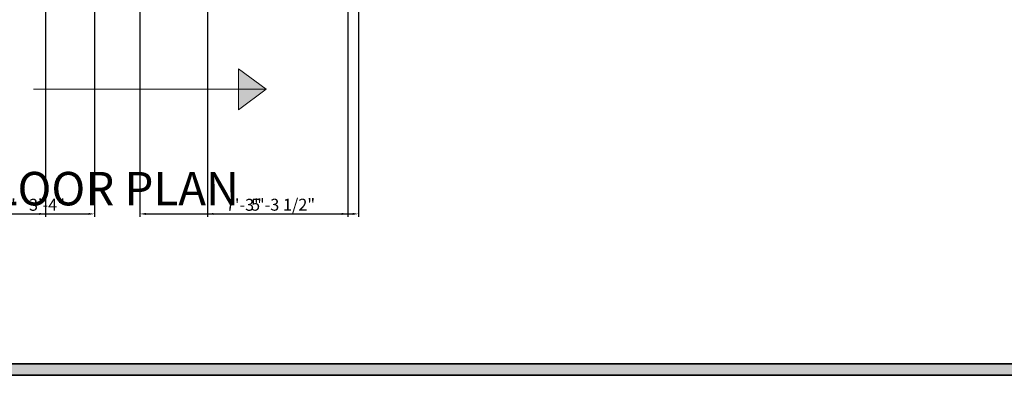
# Model space of a CAD drawing. Units: inches. Extents: x 1804 to 3296, y 909 to 2477.
# Tile 5 of 31: x 2130 to 2543, y 909 to 1059. Entities that reach past the tile are written whole.
import ezdxf

# ---------------------------------------------------------------- set-up
doc = ezdxf.new("R2010")
doc.units = ezdxf.units.IN
for name, color, linetype, lineweight in [('A-ANNO-DIMS', 2, 'Continuous', 18), ('A-ANNO-SYMB', 7, 'Continuous', 18), ('A-ANNO-TTLB', 156, 'Continuous', 35), ('A-WALL-PATT', 10, 'Continuous', 13), ('TEXT', 190, 'Continuous', 18)]:
    doc.layers.add(name, color=color, linetype=linetype, lineweight=lineweight)
doc.styles.get("Standard").update_dxf_attribs({"font": 'arial.ttf'})
doc.dimstyles.new('ISO-25', dxfattribs={"dimtxt": 5, "dimasz": 2.5, "dimexe": 1.25, "dimexo": 0.625, "dimtad": 1, "dimdec": 0, "dimlunit": 4, "dimtxsty": 'Standard', "dimcen": 2.5, "dimadec": 0, "dimazin": 0, "dimtfac": 1, "dimtdec": 0, "dimtmove": 0, "dimatfit": 3, "dimfxl": 1, "dimarcsym": 0})

# ---------------------------------------------------------------- blocks, each defined once
blk = doc.blocks.new('ROAD-DIRECTION')
h = blk.add_hatch(color=256)
h.dxf.hatch_style = 1
h.paths.add_polyline_path([(11.63, 8.56), (0, 8.56), (11.63, 0)])
h.paths.add_polyline_path([(11.63, 17.12), (0, 8.56), (11.63, 8.56)])
for p, q in [((0, 8.56), (11.63, 17.12)), ((11.63, 0), (11.63, 17.12)), ((97.65, 8.56), (0, 8.56)), ((0, 8.56), (11.63, 0))]:
    blk.add_line(p, q)
blk = doc.blocks.new('*D56')
at = {"layer": 'A-ANNO-DIMS', "color": 0, "lineweight": -2, "transparency": 16777216}
for p, q in [((2180.87, 1680.42), (2180.87, 975.89)), ((2268, 1680.42), (2268, 975.89)), ((2183.37, 977.14), (2265.5, 977.14))]:
    blk.add_line(p, q, dxfattribs=at)
at = {"layer": 'A-ANNO-DIMS', "color": 0, "lineweight": 100, "transparency": 16777216}
for points in [[(2183.37, 977.56), (2183.37, 976.72), (2180.87, 977.14)], [(2265.5, 977.56), (2265.5, 976.72), (2268, 977.14)]]:
    blk.add_solid(points, dxfattribs=at)
at = {"layer": 'Defpoints', "color": 0, "lineweight": 100, "transparency": 16777216}
for p in [(2180.87, 1681.04), (2268, 1681.04), (2268, 977.14)]:
    blk.add_point(p, dxfattribs=at)
at = {"layer": 'A-ANNO-DIMS', "color": 0, "transparency": 16777216, "insert": (2224.44, 980.32), "char_height": 5, "attachment_point": 5}
blk.add_mtext('7\'-3"', dxfattribs=at)
blk = doc.blocks.new('*D59')
at = {"layer": 'A-ANNO-DIMS', "color": 0, "lineweight": -2, "transparency": 16777216}
for p, q in [((2121.83, 1590.3), (2121.83, 975.89)), ((2161.83, 1590.3), (2161.83, 975.89)), ((2124.33, 977.14), (2159.33, 977.14))]:
    blk.add_line(p, q, dxfattribs=at)
at = {"layer": 'A-ANNO-DIMS', "color": 0, "lineweight": 100, "transparency": 16777216}
for points in [[(2124.33, 977.56), (2124.33, 976.72), (2121.83, 977.14)], [(2159.33, 977.56), (2159.33, 976.72), (2161.83, 977.14)]]:
    blk.add_solid(points, dxfattribs=at)
at = {"layer": 'Defpoints', "color": 0, "lineweight": 100, "transparency": 16777216}
for p in [(2121.83, 1590.92), (2161.83, 1590.92), (2161.83, 977.14)]:
    blk.add_point(p, dxfattribs=at)
at = {"layer": 'A-ANNO-DIMS', "color": 0, "transparency": 16777216, "insert": (2141.83, 980.32), "char_height": 5, "attachment_point": 5}
blk.add_mtext('3\'-4"', dxfattribs=at)
blk = doc.blocks.new('*D61')
at = {"layer": 'A-ANNO-DIMS', "color": 0, "lineweight": -2, "transparency": 16777216}
for p, q in [((2101.21, 1137.44), (2101.21, 975.89)), ((2141.21, 1137.44), (2141.21, 975.89)), ((2103.71, 977.14), (2138.71, 977.14))]:
    blk.add_line(p, q, dxfattribs=at)
at = {"layer": 'A-ANNO-DIMS', "color": 0, "lineweight": 100, "transparency": 16777216}
for points in [[(2103.71, 977.56), (2103.71, 976.72), (2101.21, 977.14)], [(2138.71, 977.56), (2138.71, 976.72), (2141.21, 977.14)]]:
    blk.add_solid(points, dxfattribs=at)
at = {"layer": 'Defpoints', "color": 0, "lineweight": 100, "transparency": 16777216}
for p in [(2101.21, 1138.07), (2141.21, 1138.07), (2141.21, 977.14)]:
    blk.add_point(p, dxfattribs=at)
at = {"layer": 'A-ANNO-DIMS', "color": 0, "transparency": 16777216, "insert": (2121.21, 980.32), "char_height": 5, "attachment_point": 5}
blk.add_mtext('3\'-4"', dxfattribs=at)
blk = doc.blocks.new('*D69')
at = {"layer": 'A-ANNO-DIMS', "color": 0, "lineweight": -2, "transparency": 16777216}
for p, q in [((2209.19, 1223.01), (2209.19, 975.89)), ((2272.59, 1223.01), (2272.59, 975.89)), ((2211.69, 977.14), (2270.09, 977.14))]:
    blk.add_line(p, q, dxfattribs=at)
at = {"layer": 'A-ANNO-DIMS', "color": 0, "lineweight": 100, "transparency": 16777216}
for points in [[(2211.69, 977.56), (2211.69, 976.72), (2209.19, 977.14)], [(2270.09, 977.56), (2270.09, 976.72), (2272.59, 977.14)]]:
    blk.add_solid(points, dxfattribs=at)
at = {"layer": 'Defpoints', "color": 0, "lineweight": 100, "transparency": 16777216}
for p in [(2209.19, 1223.63), (2272.59, 1223.63), (2272.59, 977.14)]:
    blk.add_point(p, dxfattribs=at)
at = {"layer": 'A-ANNO-DIMS', "color": 0, "transparency": 16777216, "insert": (2240.89, 980.35), "char_height": 5, "attachment_point": 5}
blk.add_mtext('5\'-3 1/2"', dxfattribs=at)

msp = doc.modelspace()

# ---------------------------------------------------------------- hatches: boundary and pattern name
at = {"layer": 'A-ANNO-TTLB'}
h = msp.add_hatch(color=256, dxfattribs=at)
h.dxf.hatch_style = 1
h.paths.add_polyline_path([(3294.53, 2476.54), (1803.79, 2476.54), (1805.43, 909.47), (3296.17, 909.47)])
h.paths.add_polyline_path([(1811, 914.33), (1812.79, 2467.54), (3285.53, 2467.54), (3283.74, 914.33)], flags=16)
h.paths.add_polyline_path([(1925.58, 1062.77), (1925.58, 1138.07), (1925.58, 1539.88), (1925.58, 1793.38), (1925.58, 1830.04), (2325.54, 1830.04), (2325.54, 1793.38), (2325.54, 1586.42), (2325.54, 1138.07), (2325.54, 1062.77)], flags=0)
h.paths.add_polyline_path([(1997.22, 1029.4), (2008.85, 1037.96), (2008.85, 1020.84)], flags=0)
h.paths.add_polyline_path([(1934.58, 1138.07), (1934.58, 1147.07), (2078.77, 1147.07), (2078.77, 1138.07), (2060.94, 1138.07)], flags=0)
h.paths.add_polyline_path([(1944.35, 1138.07), (1944.35, 1147.07), (2056.05, 1147.07), (2056.05, 1138.07)], flags=0)
h.paths.add_polyline_path([(2222.24, 1037.96), (2233.87, 1029.4), (2222.24, 1020.84)], flags=0)
h.paths.add_polyline_path([(2061.94, 1139.07), (2061.94, 1146.07), (2077.77, 1146.07), (2077.77, 1139.07)], flags=0)
h.paths.add_polyline_path([(2149.58, 1138.07), (2149.58, 1269.44), (2158.58, 1269.44), (2158.58, 1326.69), (2149.58, 1326.69), (2149.58, 1340.94), (2139.6, 1340.94), (2139.6, 1434.25), (2149.58, 1434.25), (2149.58, 1447.36), (2158.58, 1447.36), (2158.58, 1423.87), (2158.58, 1408.06), (2198.46, 1408.06), (2198.46, 1412.56), (2282.65, 1412.56), (2282.65, 1465.94), (2316.54, 1465.94), (2316.54, 1590.92), (2192.86, 1590.92), (2192.86, 1595.3), (2291.17, 1595.3), (2291.17, 1590.92), (2316.54, 1590.92), (2316.54, 1784.38), (2300.24, 1784.38), (2300.24, 1757.47), (2268, 1757.47), (2268, 1681.04), (2180.87, 1681.04), (2180.87, 1757.47), (2148.63, 1757.47), (2148.63, 1784.38), (2119.08, 1784.38), (2119.08, 1585.58), (2114.58, 1585.58), (2114.58, 1784.38), (2064.11, 1784.38), (2046.28, 1784.38), (2046.28, 1760.38), (1958.58, 1760.38), (1958.58, 1664.38), (1934.58, 1664.38), (1934.58, 1784.38), (1934.58, 1793.38), (2046.28, 1793.38), (2064.11, 1793.38), (2119.08, 1793.38), (2230.78, 1793.38), (2230.78, 1784.38), (2268, 1784.38), (2300.24, 1784.38), (2316.54, 1784.38), (2316.54, 1590.92), (2316.54, 1373.73), (2316.54, 1138.07)], flags=0)
h.paths.add_polyline_path([(2209.19, 1166.63), (2209.19, 1175.63), (2158.58, 1175.63), (2209.19, 1223.63), (2209.19, 1231.63), (2183.88, 1231.63), (2183.88, 1301.66), (2242.59, 1301.66), (2242.59, 1326.69), (2316.54, 1326.69), (2272.59, 1271.63), (2272.59, 1223.63), (2316.54, 1175.63), (2272.59, 1175.63), (2272.59, 1166.63)], flags=0)
h.paths.add_polyline_path([(1947.77, 1345.22), (1947.77, 1457.48), (1991.2, 1457.48), (1991.2, 1451.7), (1991.2, 1352.18), (1991.2, 1345.22)], flags=0)
h.paths.add_polyline_path([(2209.19, 1271.63), (2262.59, 1271.63), (2262.59, 1311.85), (2272.59, 1301.66), (2272.59, 1271.63), (2269.92, 1269.63), (2270.59, 1269.63), (2270.59, 1225.63), (2211.19, 1225.63), (2211.19, 1269.63), (2211.86, 1269.63)], flags=0)
h.paths.add_polyline_path([(2000.34, 1378.21), (2000.34, 1429.71), (2025.22, 1429.71), (2025.22, 1378.21)], flags=0)
h.paths.add_polyline_path([(2001.34, 1379.21), (2001.34, 1428.71), (2024.22, 1428.71), (2024.22, 1379.21)], flags=0)
h.paths.add_polyline_path([(2012.34, 1390.21), (2012.34, 1417.71), (2013.22, 1417.71), (2013.22, 1390.21)], flags=0)
h.paths.add_polyline_path([(2237.56, 1331.19), (2237.56, 1340.18), (2238.62, 1340.18), (2238.62, 1386.84), (2241.04, 1386.84), (2242.06, 1386.84), (2242.06, 1408.06), (2316.54, 1331.19)], flags=0)
h.paths.add_polyline_path([(1953.73, 1464.35), (1953.73, 1498.59), (1981.74, 1498.59), (1981.74, 1464.35)], flags=0)
h.paths.add_polyline_path([(1987.63, 1462.08), (1987.63, 1500.95), (2104.07, 1500.95), (2104.07, 1462.08), (2099.27, 1462.08), (1993.6, 1462.08)], flags=0)
h.paths.add_polyline_path([(1956.06, 1481.47, -1), (1979.41, 1481.47, -1)], flags=0)
edge = h.paths.add_edge_path(flags=0)
edge.add_ellipse((2299.53, 1438.37), major_axis=(0.31, 21.36), ratio=0.670333, start_angle=0, end_angle=360)
h.paths.add_polyline_path([(2297.39, 1438.37, -1), (2301.67, 1438.37, -1)], flags=0)
h.paths.add_polyline_path([(2591.54, 1163.23), (2591.54, 1179.38), (2591.54, 1379.68), (2591.54, 1395.84), (2734.5, 1395.84), (2734.5, 1379.68), (2734.5, 1179.38), (2734.5, 1163.23)], flags=0)
h.paths.add_polyline_path([(2592.54, 1164.23), (2592.54, 1166.23), (2733.5, 1166.23), (2733.5, 1164.23)], flags=0)
h.paths.add_polyline_path([(2592.54, 1180.38), (2592.54, 1378.68), (2733.5, 1378.68), (2733.5, 1180.38)], flags=0)
h.paths.add_polyline_path([(2593.54, 1181.38), (2593.54, 1377.68), (2732.5, 1377.68), (2732.5, 1181.38)], flags=0)
h.paths.add_polyline_path([(2594.54, 1182.38), (2594.54, 1376.68), (2731.5, 1376.68), (2731.5, 1182.38)], flags=0)
h.paths.add_polyline_path([(1936.95, 1697.46), (1936.95, 1736.46), (1955.41, 1736.46), (1955.41, 1697.46)], flags=0)
h.paths.add_polyline_path([(1938.48, 1718.36), (1938.48, 1734.92), (1953.65, 1734.92), (1953.65, 1718.36)], flags=0)
h.paths.add_polyline_path([(1944.75, 1726.64, -1), (1947.37, 1726.64, -1)], flags=0)
h.paths.add_polyline_path([(2592.54, 1394.84), (2733.5, 1394.84), (2733.5, 1392.84), (2592.54, 1392.84)], flags=0)
h.paths.add_polyline_path([(1976.61, 1762.5), (1976.61, 1781.44), (2012.79, 1781.44), (2012.79, 1762.5)], flags=0)
h.paths.add_polyline_path([(1979.57, 1771.97, -1), (1991.39, 1771.97, -1)], flags=0)
h.paths.add_polyline_path([(1995.36, 1771.97, -1), (2007.18, 1771.97, -1)], flags=0)
h.paths.add_polyline_path([(2251.51, 1744.53), (2268, 1730.05), (2251.51, 1730.05)], flags=0)
h.paths.add_polyline_path([(2047.28, 1785.38), (2047.28, 1792.38), (2063.11, 1792.38), (2063.11, 1785.38)], flags=0)
h.paths.add_polyline_path([(2155.08, 1770.92, -1), (2174.42, 1770.92, -1)], flags=0)
h.paths.add_polyline_path([(2188.59, 1758.27), (2188.59, 1772.81), (2222.3, 1772.81), (2222.3, 1758.27)], flags=0)
h.paths.add_polyline_path([(2223.97, 1758.27), (2223.97, 1772.81), (2257.68, 1772.81), (2257.68, 1758.27)], flags=0)
h.paths.add_polyline_path([(2274.45, 1770.92, -1), (2293.8, 1770.92, -1)], flags=0)
h.paths.add_polyline_path([(2591.54, 1582.09), (2591.54, 1782.39), (2734.5, 1782.39), (2734.5, 1582.09)], flags=0)
h.paths.add_polyline_path([(2592.54, 1583.09), (2592.54, 1781.39), (2733.5, 1781.39), (2733.5, 1583.09)], flags=0)
h.paths.add_polyline_path([(2593.54, 1584.09), (2593.54, 1780.39), (2732.5, 1780.39), (2732.5, 1584.09)], flags=0)
h.paths.add_polyline_path([(2594.54, 1585.09), (2594.54, 1779.39), (2731.5, 1779.39), (2731.5, 1585.09)], flags=0)
h.paths.add_polyline_path([(1922.17, 1978.79), (1922.17, 2295.08), (1922.17, 2296.08), (2115.67, 2296.08), (2115.67, 2384.31), (2115.67, 2385.31), (2322.12, 2385.31), (2323.12, 2385.31), (2323.12, 1979.79), (2323.12, 1978.79), (1923.17, 1978.79)], flags=0)
h.paths.add_polyline_path([(1922.17, 1978.79), (1922.17, 2051.31), (1922.17, 2214.86), (1922.17, 2296.08), (2115.67, 2296.08), (2115.67, 2385.31), (2323.12, 2385.31), (2323.12, 2280.42), (2323.12, 1978.79), (2115.67, 1978.79)], flags=0)
h.paths.add_polyline_path([(1923.17, 1979.79), (1923.17, 2050.31), (2115.67, 2050.31), (2115.67, 2051.31), (1923.17, 2051.31), (1923.17, 2213.86), (1923.17, 2214.86), (1923.17, 2295.08), (1990.02, 2295.08), (1990.02, 2214.86), (1991.02, 2214.86), (1991.02, 2295.08), (2115.67, 2295.08), (2115.67, 1979.79), (2116.67, 1979.79), (2116.67, 2304.18), (2116.67, 2384.31), (2322.12, 2384.31), (2322.12, 2280.42), (2322.12, 1979.79), (2115.67, 1979.79)], flags=0)
h.paths.add_polyline_path([(2972.46, 1192.5), (2972.46, 1196.92), (2995.47, 1196.92), (2995.47, 1255.47), (2995.09, 1255.47), (2987.42, 1249.39), (2980.08, 1255.47), (2978.05, 1255.47), (2978.05, 1257.24), (2995.47, 1257.24), (2995.47, 1261.58), (3015.37, 1261.58), (3015.37, 1333.28), (3015.37, 1414.4), (3032.82, 1414.4), (3032.82, 1333.28), (3032.82, 1261.58), (3052.66, 1261.58), (3052.66, 1255.47), (3079.86, 1255.47), (3078.72, 1254.57), (3081.47, 1252.29), (3078.56, 1249.99), (3075.81, 1252.26), (3072.57, 1249.69), (3070.36, 1251.52), (3067.67, 1249.39), (3060.34, 1255.47), (3052.66, 1255.47), (3052.66, 1196.92), (3054.58, 1196.92), (3074, 1196.92), (3074, 1192.5), (3052.66, 1192.5), (2995.47, 1192.5)], flags=0)
h.paths.add_polyline_path([(2490.75, 1979.27), (2490.75, 1980.27), (2596.87, 1980.27), (2596.87, 2051.8), (2596.87, 2052.8), (2596.87, 2216.35), (2596.87, 2297.57), (2717.32, 2297.57), (2710.57, 2305.62), (2724.07, 2305.62), (2717.32, 2297.57), (2782.37, 2297.57), (2782.37, 2395.8), (3006.82, 2395.8), (3006.82, 1981.27), (3093.73, 1981.27), (3093.73, 1980.27), (3047.51, 1980.27), (3046.37, 1979.37), (3049.11, 1977.1), (3046.2, 1974.79), (3043.46, 1977.07), (3040.21, 1974.49), (3038, 1976.32), (3035.32, 1974.2), (3027.98, 1980.27), (2871.83, 1980.27), (2871.83, 1981.27), (2791.37, 1981.27), (2791.37, 2050.8), (2597.87, 2050.8), (2597.87, 1980.27), (2597.87, 1979.27), (2546.27, 1979.27), (2545.12, 1978.37), (2547.87, 1976.1), (2544.96, 1973.79), (2542.22, 1976.07), (2538.97, 1973.49), (2536.76, 1975.32), (2534.07, 1973.2), (2526.74, 1979.27)], flags=0)
h.paths.add_polyline_path([(2597.87, 2051.8), (2606.87, 2051.8), (2606.87, 2258.39), (2597.87, 2258.39), (2597.87, 2296.57), (2606.87, 2296.57), (2606.87, 2262.39), (2782.37, 2262.39), (2782.37, 2296.57), (2790.37, 2296.57), (2790.37, 2262.39), (2791.37, 2262.39), (2791.37, 2305.67), (2791.37, 2385.8), (2996.82, 2385.8), (2996.82, 2339.85), (3006.82, 2339.85), (3006.82, 2250.12), (2997.82, 2250.12), (2997.82, 1981.27), (2996.82, 1981.27), (2872.83, 1981.27), (2872.83, 1991.8), (2871.83, 1991.8), (2871.83, 2050.8), (2790.37, 2050.8), (2597.87, 2050.8)], flags=0)
h.paths.add_polyline_path([(2179.93, 2153.92), (2179.93, 2353.97), (2259.98, 2353.97), (2259.98, 2153.92)], flags=0)
h.paths.add_polyline_path([(2180.93, 2154.92), (2180.93, 2352.97), (2258.98, 2352.97), (2258.98, 2154.92)], flags=0)
h.paths.add_polyline_path([(2960.87, 1608.49), (2960.87, 1753.62), (3070.9, 1753.62), (3070.9, 1608.49)], flags=0)
h.paths.add_polyline_path([(2961.87, 1609.49), (2961.87, 1752.62), (3069.9, 1752.62), (3069.9, 1609.49)], flags=0)
h.paths.add_polyline_path([(2962.87, 1610.49), (2962.87, 1751.62), (3068.9, 1751.62), (3068.9, 1610.49)], flags=0)
h.paths.add_polyline_path([(2963.87, 1611.49), (2963.87, 1750.62), (3067.9, 1750.62), (3067.9, 1611.49)], flags=0)
h.paths.add_polyline_path([(2782.37, 2051.8), (2782.37, 2216.32), (2791.37, 2216.32), (2791.37, 2051.8), (2872.83, 2051.8), (2872.83, 2068.56), (2884.67, 2068.56), (2884.67, 2085.33), (2896.51, 2085.33), (2896.51, 2102.09), (2908.36, 2102.09), (2908.36, 2118.85), (2920.2, 2118.85), (2920.2, 2135.62), (2932.05, 2135.62), (2932.05, 2145.3), (2925.08, 2145.3), (2925.08, 2203.2), (2996.82, 2203.2), (2996.82, 2145.3), (2953.82, 2145.3), (2872.83, 2051.8), (2790.37, 2051.8)], flags=0)
h.paths.add_polyline_path([(2717.32, 2238.65), (2710.57, 2246.7), (2724.07, 2246.7)], flags=0)
h.paths.add_polyline_path([(2003.09, 1122.79), (2017.16, 1122.79), (2017.16, 1138.74), (2003.09, 1138.74)], flags=8)
h.paths.add_polyline_path([(2174.76, 1792.72), (2188.83, 1792.72), (2188.83, 1808.66), (2174.76, 1808.66)], flags=8)
h.paths.add_polyline_path([(1987.95, 1792.51), (2002.02, 1792.51), (2002.02, 1808.45), (1987.95, 1808.45)], flags=8)
h.paths.add_polyline_path([(2148.79, 1289.26), (2160.46, 1289.26), (2160.46, 1305.2), (2148.79, 1305.2)], flags=8)
h.paths.add_polyline_path([(2115.36, 1133.57), (2127.04, 1133.57), (2127.04, 1149.51), (2115.36, 1149.51)], flags=8)
h.paths.add_polyline_path([(2237.58, 1421.48), (2249.25, 1421.48), (2249.25, 1437.43), (2237.58, 1437.43)], flags=8)
h.paths.add_polyline_path([(2134.99, 1584.32), (2146.66, 1584.32), (2146.66, 1600.26), (2134.99, 1600.26)], flags=8)
h.paths.add_polyline_path([(2101.95, 1557.31), (2113.62, 1557.31), (2113.62, 1573.25), (2101.95, 1573.25)], flags=8)
h.paths.add_polyline_path([(2937.85, 1156.77), (3120.41, 1156.77), (3120.41, 1185.72), (2937.85, 1185.72)], flags=8)
h.paths.add_polyline_path([(2980.71, 1786.71), (3050.06, 1786.71), (3050.06, 1802.66), (2980.71, 1802.66)], flags=8)
h.paths.add_polyline_path([(2869.28, 1661.96), (2938.62, 1661.96), (2938.62, 1690.8), (2869.28, 1690.8)], flags=8)
h.paths.add_polyline_path([(3092.27, 1674.86), (3161.62, 1674.86), (3161.62, 1690.8), (3092.27, 1690.8)], flags=8)
h.paths.add_polyline_path([(2980.71, 1674.86), (3050.06, 1674.86), (3050.06, 1690.8), (2980.71, 1690.8)], flags=8)
h.paths.add_polyline_path([(2649.07, 1678.23), (2674.53, 1678.23), (2674.53, 1714.76), (2649.07, 1714.76)], flags=8)
h.paths.add_polyline_path([(2530.84, 1981.63), (2549.13, 1981.63), (2549.13, 1997.57), (2530.84, 1997.57)], flags=8)
h.paths.add_polyline_path([(3031.29, 1981.77), (3049.58, 1981.77), (3049.58, 1997.71), (3031.29, 1997.71)], flags=8)
h.paths.add_polyline_path([(2715.38, 1911.9), (2851.54, 1911.9), (2851.54, 1940.85), (2715.38, 1940.85)], flags=8)
h.paths.add_polyline_path([(2015.23, 1927.36), (2205.42, 1927.36), (2205.42, 1956.3), (2015.23, 1956.3)], flags=8)
h.paths.add_polyline_path([(2671.84, 2057.84), (2702.75, 2057.84), (2702.75, 2073.79), (2671.84, 2073.79)], flags=8)
h.paths.add_polyline_path([(2678.5, 2316.52), (2765.26, 2316.52), (2765.26, 2332.46), (2678.5, 2332.46)], flags=8)
h.paths.add_polyline_path([(2678.48, 2271.96), (2736.41, 2271.96), (2736.41, 2287.9), (2678.48, 2287.9)], flags=8)
h.paths.add_polyline_path([(2019.2, 972.79), (2243.21, 972.79), (2243.21, 1001.74), (2019.2, 1001.74)], flags=8)
h.paths.add_polyline_path([(2097.06, 1021.56), (2132.16, 1021.56), (2132.16, 1037.51), (2097.06, 1037.51)], flags=8)
h.paths.add_polyline_path([(2182.47, 1360.48), (2207.35, 1360.48), (2207.35, 1376.42), (2182.47, 1376.42)], flags=8)
h.paths.add_polyline_path([(2261.12, 1361.77), (2295.01, 1361.77), (2295.01, 1377.71), (2261.12, 1377.71)], flags=8)
h.paths.add_polyline_path([(2245.75, 1511.51), (2278.44, 1511.51), (2278.44, 1527.46), (2245.75, 1527.46)], flags=8)
h.paths.add_polyline_path([(1991.16, 1296.29), (2060.51, 1296.29), (2060.51, 1312.23), (1991.16, 1312.23)], flags=8)
h.paths.add_polyline_path([(2187, 1651.35), (2246.71, 1651.35), (2246.71, 1667.29), (2187, 1667.29)], flags=8)
h.paths.add_polyline_path([(1976.49, 1684.81), (2068.63, 1684.81), (2068.63, 1700.76), (1976.49, 1700.76)], flags=8)
at = {"layer": 'A-WALL-PATT'}
h = msp.add_hatch(color=256, dxfattribs=at)
h.dxf.hatch_style = 1
h.paths.add_polyline_path([(2119.08, 1544.38), (1925.58, 1544.38), (1925.58, 1539.88), (2119.08, 1539.88)])
h.paths.add_polyline_path([(2119.08, 1545.58), (2114.58, 1545.58), (2114.58, 1544.38), (2119.08, 1544.38)])
h.paths.add_polyline_path([(1965.87, 1658.79), (1965.87, 1679.09), (1955.57, 1679.09), (1955.57, 1658.79)], flags=9)
h.paths.add_polyline_path([(2293.18, 1677.29), (2293.18, 1697.58), (2282.88, 1697.58), (2282.88, 1677.29)], flags=9)
h.paths.add_polyline_path([(2271.13, 1545.23), (2287.53, 1545.23), (2287.53, 1555.53), (2271.13, 1555.53)], flags=9)
h.paths.add_polyline_path([(2303.26, 1488.52), (2303.26, 1508.82), (2292.95, 1508.82), (2292.95, 1488.52)], flags=9)
h.paths.add_polyline_path([(2271.13, 1393.15), (2287.53, 1393.15), (2287.53, 1403.45), (2271.13, 1403.45)], flags=9)
h.paths.add_polyline_path([(2306.48, 1361.45), (2306.48, 1377.86), (2296.18, 1377.86), (2296.18, 1361.45)], flags=9)
h.paths.add_polyline_path([(2174.54, 1361.45), (2174.54, 1377.86), (2164.23, 1377.86), (2164.23, 1361.45)], flags=9)
h.paths.add_polyline_path([(1968.21, 1333.34), (1968.21, 1353.64), (1957.91, 1353.64), (1957.91, 1333.34)], flags=9)
h.paths.add_polyline_path([(2003.09, 1122.79), (2017.16, 1122.79), (2017.16, 1138.74), (2003.09, 1138.74)], flags=9)
h.paths.add_polyline_path([(2174.76, 1792.72), (2188.83, 1792.72), (2188.83, 1808.66), (2174.76, 1808.66)], flags=9)
h.paths.add_polyline_path([(1987.95, 1792.51), (2002.02, 1792.51), (2002.02, 1808.45), (1987.95, 1808.45)], flags=9)
h.paths.add_polyline_path([(2148.79, 1289.26), (2160.46, 1289.26), (2160.46, 1305.2), (2148.79, 1305.2)], flags=9)
h.paths.add_polyline_path([(2115.36, 1133.57), (2127.04, 1133.57), (2127.04, 1149.51), (2115.36, 1149.51)], flags=9)
h.paths.add_polyline_path([(2237.58, 1421.48), (2249.25, 1421.48), (2249.25, 1437.43), (2237.58, 1437.43)], flags=9)
h.paths.add_polyline_path([(2134.99, 1584.32), (2146.66, 1584.32), (2146.66, 1600.26), (2134.99, 1600.26)], flags=9)
h.paths.add_polyline_path([(2101.95, 1557.31), (2113.62, 1557.31), (2113.62, 1573.25), (2101.95, 1573.25)], flags=9)
h.paths.add_polyline_path([(2937.85, 1156.77), (3120.41, 1156.77), (3120.41, 1185.72), (2937.85, 1185.72)], flags=9)
h.paths.add_polyline_path([(2980.71, 1786.71), (3050.06, 1786.71), (3050.06, 1802.66), (2980.71, 1802.66)], flags=9)
h.paths.add_polyline_path([(2869.28, 1661.96), (2938.62, 1661.96), (2938.62, 1690.8), (2869.28, 1690.8)], flags=9)
h.paths.add_polyline_path([(3092.27, 1674.86), (3161.62, 1674.86), (3161.62, 1690.8), (3092.27, 1690.8)], flags=9)
h.paths.add_polyline_path([(2980.71, 1674.86), (3050.06, 1674.86), (3050.06, 1690.8), (2980.71, 1690.8)], flags=9)
h.paths.add_polyline_path([(2649.07, 1678.23), (2674.53, 1678.23), (2674.53, 1714.76), (2649.07, 1714.76)], flags=9)
h.paths.add_polyline_path([(2530.84, 1981.63), (2549.13, 1981.63), (2549.13, 1997.57), (2530.84, 1997.57)], flags=9)
h.paths.add_polyline_path([(3031.29, 1981.77), (3049.58, 1981.77), (3049.58, 1997.71), (3031.29, 1997.71)], flags=9)
h.paths.add_polyline_path([(2715.38, 1911.9), (2851.54, 1911.9), (2851.54, 1940.85), (2715.38, 1940.85)], flags=9)
h.paths.add_polyline_path([(2015.23, 1927.36), (2205.42, 1927.36), (2205.42, 1956.3), (2015.23, 1956.3)], flags=9)
h.paths.add_polyline_path([(2671.84, 2057.84), (2702.75, 2057.84), (2702.75, 2073.79), (2671.84, 2073.79)], flags=9)
h.paths.add_polyline_path([(2678.5, 2316.52), (2765.26, 2316.52), (2765.26, 2332.46), (2678.5, 2332.46)], flags=9)
h.paths.add_polyline_path([(2678.48, 2271.96), (2736.41, 2271.96), (2736.41, 2287.9), (2678.48, 2287.9)], flags=9)
h.paths.add_polyline_path([(2019.2, 972.79), (2243.21, 972.79), (2243.21, 1001.74), (2019.2, 1001.74)], flags=9)
h.paths.add_polyline_path([(2097.06, 1021.56), (2132.16, 1021.56), (2132.16, 1037.51), (2097.06, 1037.51)], flags=9)
h.paths.add_polyline_path([(2182.47, 1360.48), (2207.35, 1360.48), (2207.35, 1376.42), (2182.47, 1376.42)], flags=9)
h.paths.add_polyline_path([(2261.12, 1361.77), (2295.01, 1361.77), (2295.01, 1377.71), (2261.12, 1377.71)], flags=9)
h.paths.add_polyline_path([(2245.75, 1511.51), (2278.44, 1511.51), (2278.44, 1527.46), (2245.75, 1527.46)], flags=9)
h.paths.add_polyline_path([(1991.16, 1296.29), (2060.51, 1296.29), (2060.51, 1312.23), (1991.16, 1312.23)], flags=9)
h.paths.add_polyline_path([(2187, 1651.35), (2246.71, 1651.35), (2246.71, 1667.29), (2187, 1667.29)], flags=9)
h.paths.add_polyline_path([(1976.49, 1684.81), (2068.63, 1684.81), (2068.63, 1700.76), (1976.49, 1700.76)], flags=9)
h = msp.add_hatch(color=256, dxfattribs=at)
h.dxf.hatch_style = 1
h.paths.add_polyline_path([(2149.58, 1147.07), (2141.21, 1147.07), (2141.21, 1144.07), (2141.21, 1138.07), (2149.58, 1138.07)])
h.paths.add_polyline_path([(2101.21, 1144.07, -0.01877), (2101.32, 1147.07), (2078.77, 1147.07), (2078.77, 1138.07), (2101.21, 1138.07)])
h.paths.add_polyline_path([(2060.94, 1147.07), (2056.05, 1147.07), (2056.05, 1138.07), (2060.94, 1138.07)])
h.paths.add_polyline_path([(1944.35, 1147.07), (1934.58, 1147.07), (1934.58, 1138.07), (1944.35, 1138.07)])
h.paths.add_polyline_path([(2158.58, 1269.44), (2149.58, 1269.44), (2149.58, 1138.07), (2158.58, 1138.07)])
h.paths.add_polyline_path([(2003.09, 1122.79), (2017.16, 1122.79), (2017.16, 1138.74), (2003.09, 1138.74)], flags=9)
h.paths.add_polyline_path([(2174.76, 1792.72), (2188.83, 1792.72), (2188.83, 1808.66), (2174.76, 1808.66)], flags=9)
h.paths.add_polyline_path([(1987.95, 1792.51), (2002.02, 1792.51), (2002.02, 1808.45), (1987.95, 1808.45)], flags=9)
h.paths.add_polyline_path([(2148.79, 1289.26), (2160.46, 1289.26), (2160.46, 1305.2), (2148.79, 1305.2)], flags=9)
h.paths.add_polyline_path([(2115.36, 1133.57), (2127.04, 1133.57), (2127.04, 1149.51), (2115.36, 1149.51)], flags=9)
h.paths.add_polyline_path([(2237.58, 1421.48), (2249.25, 1421.48), (2249.25, 1437.43), (2237.58, 1437.43)], flags=9)
h.paths.add_polyline_path([(2134.99, 1584.32), (2146.66, 1584.32), (2146.66, 1600.26), (2134.99, 1600.26)], flags=9)
h.paths.add_polyline_path([(2101.95, 1557.31), (2113.62, 1557.31), (2113.62, 1573.25), (2101.95, 1573.25)], flags=9)
h.paths.add_polyline_path([(2937.85, 1156.77), (3120.41, 1156.77), (3120.41, 1185.72), (2937.85, 1185.72)], flags=9)
h.paths.add_polyline_path([(2980.71, 1786.71), (3050.06, 1786.71), (3050.06, 1802.66), (2980.71, 1802.66)], flags=9)
h.paths.add_polyline_path([(2869.28, 1661.96), (2938.62, 1661.96), (2938.62, 1690.8), (2869.28, 1690.8)], flags=9)
h.paths.add_polyline_path([(3092.27, 1674.86), (3161.62, 1674.86), (3161.62, 1690.8), (3092.27, 1690.8)], flags=9)
h.paths.add_polyline_path([(2980.71, 1674.86), (3050.06, 1674.86), (3050.06, 1690.8), (2980.71, 1690.8)], flags=9)
h.paths.add_polyline_path([(2649.07, 1678.23), (2674.53, 1678.23), (2674.53, 1714.76), (2649.07, 1714.76)], flags=9)
h.paths.add_polyline_path([(2530.84, 1981.63), (2549.13, 1981.63), (2549.13, 1997.57), (2530.84, 1997.57)], flags=9)
h.paths.add_polyline_path([(3031.29, 1981.77), (3049.58, 1981.77), (3049.58, 1997.71), (3031.29, 1997.71)], flags=9)
h.paths.add_polyline_path([(2715.38, 1911.9), (2851.54, 1911.9), (2851.54, 1940.85), (2715.38, 1940.85)], flags=9)
h.paths.add_polyline_path([(2015.23, 1927.36), (2205.42, 1927.36), (2205.42, 1956.3), (2015.23, 1956.3)], flags=9)
h.paths.add_polyline_path([(2671.84, 2057.84), (2702.75, 2057.84), (2702.75, 2073.79), (2671.84, 2073.79)], flags=9)
h.paths.add_polyline_path([(2678.5, 2316.52), (2765.26, 2316.52), (2765.26, 2332.46), (2678.5, 2332.46)], flags=9)
h.paths.add_polyline_path([(2678.48, 2271.96), (2736.41, 2271.96), (2736.41, 2287.9), (2678.48, 2287.9)], flags=9)
h.paths.add_polyline_path([(2019.2, 972.79), (2243.21, 972.79), (2243.21, 1001.74), (2019.2, 1001.74)], flags=9)
h.paths.add_polyline_path([(2097.06, 1021.56), (2132.16, 1021.56), (2132.16, 1037.51), (2097.06, 1037.51)], flags=9)
h.paths.add_polyline_path([(2182.47, 1360.48), (2207.35, 1360.48), (2207.35, 1376.42), (2182.47, 1376.42)], flags=9)
h.paths.add_polyline_path([(2261.12, 1361.77), (2295.01, 1361.77), (2295.01, 1377.71), (2261.12, 1377.71)], flags=9)
h.paths.add_polyline_path([(2245.75, 1511.51), (2278.44, 1511.51), (2278.44, 1527.46), (2245.75, 1527.46)], flags=9)
h.paths.add_polyline_path([(1991.16, 1296.29), (2060.51, 1296.29), (2060.51, 1312.23), (1991.16, 1312.23)], flags=9)
h.paths.add_polyline_path([(2187, 1651.35), (2246.71, 1651.35), (2246.71, 1667.29), (2187, 1667.29)], flags=9)
h.paths.add_polyline_path([(1976.49, 1684.81), (2068.63, 1684.81), (2068.63, 1700.76), (1976.49, 1700.76)], flags=9)
h = msp.add_hatch(color=256, dxfattribs=at)
h.dxf.hatch_style = 1
h.paths.add_polyline_path([(2158.58, 1275.49), (2155.29, 1275.49), (2149.58, 1275.49), (2149.58, 1269.44), (2158.58, 1269.44)])
h.paths.add_polyline_path([(2158.58, 1326.69), (2149.58, 1326.69), (2149.58, 1319.33), (2155.29, 1319.33), (2158.58, 1319.33)])
h.paths.add_polyline_path([(2158.58, 1402.2), (2158.58, 1423.87), (2158.58, 1447.36), (2149.58, 1447.36), (2149.58, 1423.87), (2149.58, 1340.94), (2149.58, 1326.69), (2158.58, 1326.69), (2158.58, 1354.23)])
h.paths.add_polyline_path([(1965.87, 1658.79), (1965.87, 1679.09), (1955.57, 1679.09), (1955.57, 1658.79)], flags=9)
h.paths.add_polyline_path([(2293.18, 1677.29), (2293.18, 1697.58), (2282.88, 1697.58), (2282.88, 1677.29)], flags=9)
h.paths.add_polyline_path([(2271.13, 1545.23), (2287.53, 1545.23), (2287.53, 1555.53), (2271.13, 1555.53)], flags=9)
h.paths.add_polyline_path([(2303.26, 1488.52), (2303.26, 1508.82), (2292.95, 1508.82), (2292.95, 1488.52)], flags=9)
h.paths.add_polyline_path([(2271.13, 1393.15), (2287.53, 1393.15), (2287.53, 1403.45), (2271.13, 1403.45)], flags=9)
h.paths.add_polyline_path([(2306.48, 1361.45), (2306.48, 1377.86), (2296.18, 1377.86), (2296.18, 1361.45)], flags=9)
h.paths.add_polyline_path([(2189.9, 1340.62), (2206.31, 1340.62), (2206.31, 1350.92), (2189.9, 1350.92)], flags=9)
h.paths.add_polyline_path([(2174.54, 1361.45), (2174.54, 1377.86), (2164.23, 1377.86), (2164.23, 1361.45)], flags=9)
h.paths.add_polyline_path([(2304.24, 1240.8), (2304.24, 1261.09), (2293.94, 1261.09), (2293.94, 1240.8)], flags=9)
h.paths.add_polyline_path([(2227.19, 1188.73), (2247.49, 1188.73), (2247.49, 1199.03), (2227.19, 1199.03)], flags=9)
h.paths.add_polyline_path([(2181.93, 1144.21), (2181.93, 1160.62), (2171.63, 1160.62), (2171.63, 1144.21)], flags=9)
h.paths.add_polyline_path([(1968.21, 1333.34), (1968.21, 1353.64), (1957.91, 1353.64), (1957.91, 1333.34)], flags=9)
h.paths.add_polyline_path([(2029.78, 1203.53), (2053.95, 1203.53), (2053.95, 1213.83), (2029.78, 1213.83)], flags=9)
h.paths.add_polyline_path([(2576.51, 1671.88), (2576.51, 1692.17), (2566.21, 1692.17), (2566.21, 1671.88)], flags=9)
h.paths.add_polyline_path([(2566.99, 1269.67), (2566.99, 1289.96), (2556.68, 1289.96), (2556.68, 1269.67)], flags=9)
h.paths.add_polyline_path([(2581.85, 1269.17), (2581.85, 1289.46), (2571.54, 1289.46), (2571.54, 1269.17)], flags=9)
h.paths.add_polyline_path([(2650.71, 1409.75), (2674.89, 1409.75), (2674.89, 1420.05), (2650.71, 1420.05)], flags=9)
h.paths.add_polyline_path([(2003.09, 1122.79), (2017.16, 1122.79), (2017.16, 1138.74), (2003.09, 1138.74)], flags=9)
h.paths.add_polyline_path([(2174.76, 1792.72), (2188.83, 1792.72), (2188.83, 1808.66), (2174.76, 1808.66)], flags=9)
h.paths.add_polyline_path([(1987.95, 1792.51), (2002.02, 1792.51), (2002.02, 1808.45), (1987.95, 1808.45)], flags=9)
h.paths.add_polyline_path([(2148.79, 1289.26), (2160.46, 1289.26), (2160.46, 1305.2), (2148.79, 1305.2)], flags=9)
h.paths.add_polyline_path([(2115.36, 1133.57), (2127.04, 1133.57), (2127.04, 1149.51), (2115.36, 1149.51)], flags=9)
h.paths.add_polyline_path([(2237.58, 1421.48), (2249.25, 1421.48), (2249.25, 1437.43), (2237.58, 1437.43)], flags=9)
h.paths.add_polyline_path([(2134.99, 1584.32), (2146.66, 1584.32), (2146.66, 1600.26), (2134.99, 1600.26)], flags=9)
h.paths.add_polyline_path([(2101.95, 1557.31), (2113.62, 1557.31), (2113.62, 1573.25), (2101.95, 1573.25)], flags=9)
h.paths.add_polyline_path([(2937.85, 1156.77), (3120.41, 1156.77), (3120.41, 1185.72), (2937.85, 1185.72)], flags=9)
h.paths.add_polyline_path([(2980.71, 1786.71), (3050.06, 1786.71), (3050.06, 1802.66), (2980.71, 1802.66)], flags=9)
h.paths.add_polyline_path([(2869.28, 1661.96), (2938.62, 1661.96), (2938.62, 1690.8), (2869.28, 1690.8)], flags=9)
h.paths.add_polyline_path([(3092.27, 1674.86), (3161.62, 1674.86), (3161.62, 1690.8), (3092.27, 1690.8)], flags=9)
h.paths.add_polyline_path([(2980.71, 1674.86), (3050.06, 1674.86), (3050.06, 1690.8), (2980.71, 1690.8)], flags=9)
h.paths.add_polyline_path([(2649.07, 1678.23), (2674.53, 1678.23), (2674.53, 1714.76), (2649.07, 1714.76)], flags=9)
h.paths.add_polyline_path([(2530.84, 1981.63), (2549.13, 1981.63), (2549.13, 1997.57), (2530.84, 1997.57)], flags=9)
h.paths.add_polyline_path([(3031.29, 1981.77), (3049.58, 1981.77), (3049.58, 1997.71), (3031.29, 1997.71)], flags=9)
h.paths.add_polyline_path([(2715.38, 1911.9), (2851.54, 1911.9), (2851.54, 1940.85), (2715.38, 1940.85)], flags=9)
h.paths.add_polyline_path([(2015.23, 1927.36), (2205.42, 1927.36), (2205.42, 1956.3), (2015.23, 1956.3)], flags=9)
h.paths.add_polyline_path([(2671.84, 2057.84), (2702.75, 2057.84), (2702.75, 2073.79), (2671.84, 2073.79)], flags=9)
h.paths.add_polyline_path([(2678.5, 2316.52), (2765.26, 2316.52), (2765.26, 2332.46), (2678.5, 2332.46)], flags=9)
h.paths.add_polyline_path([(2678.48, 2271.96), (2736.41, 2271.96), (2736.41, 2287.9), (2678.48, 2287.9)], flags=9)
h.paths.add_polyline_path([(2019.2, 972.79), (2243.21, 972.79), (2243.21, 1001.74), (2019.2, 1001.74)], flags=9)
h.paths.add_polyline_path([(2097.06, 1021.56), (2132.16, 1021.56), (2132.16, 1037.51), (2097.06, 1037.51)], flags=9)
h.paths.add_polyline_path([(2182.47, 1360.48), (2207.35, 1360.48), (2207.35, 1376.42), (2182.47, 1376.42)], flags=9)
h.paths.add_polyline_path([(2261.12, 1361.77), (2295.01, 1361.77), (2295.01, 1377.71), (2261.12, 1377.71)], flags=9)
h.paths.add_polyline_path([(2245.75, 1511.51), (2278.44, 1511.51), (2278.44, 1527.46), (2245.75, 1527.46)], flags=9)
h.paths.add_polyline_path([(1991.16, 1296.29), (2060.51, 1296.29), (2060.51, 1312.23), (1991.16, 1312.23)], flags=9)
h.paths.add_polyline_path([(2187, 1651.35), (2246.71, 1651.35), (2246.71, 1667.29), (2187, 1667.29)], flags=9)
h.paths.add_polyline_path([(1976.49, 1684.81), (2068.63, 1684.81), (2068.63, 1700.76), (1976.49, 1700.76)], flags=9)

# ---------------------------------------------------------------- linework, layer by layer
at = {"layer": 'A-ANNO-TTLB'}
for points in [[(1803.79, 2476.54), (3294.53, 2476.54), (3296.17, 909.47), (1805.43, 909.47)], [(1812.79, 2467.54), (3285.53, 2467.54), (3283.74, 914.33), (1811, 914.33)]]:
    msp.add_lwpolyline(points, close=True, dxfattribs=at)

# ---------------------------------------------------------------- block references
at = {"layer": 'A-ANNO-SYMB', "extrusion": (0, 0, -1), "zscale": -1}
msp.add_blockref('ROAD-DIRECTION', (-2233.87, 1020.84), dxfattribs=at)

# ---------------------------------------------------------------- texts
at = {"layer": 'TEXT', "insert": (2023.76, 994.76), "char_height": 14.0468, "attachment_point": 1}
msp.add_mtext_dynamic_manual_height_columns('GROUND FLOOR PLAN', width=296.512, gutter_width=70.23, heights=[0], dxfattribs=at)

# ---------------------------------------------------------------- dimensions: what is measured, and where the dimension line sits
at = {"layer": 'A-ANNO-DIMS'}
for base, p1, p2, picture, middle in [((2268, 977.14), (2180.87, 1681.04), (2268, 1681.04), '*D56', (2224.44, 980.32)), ((2161.83, 977.14), (2121.83, 1590.92), (2161.83, 1590.92), '*D59', (2141.83, 980.32)), ((2272.59, 977.14), (2209.19, 1223.63), (2272.59, 1223.63), '*D69', (2240.89, 980.35)), ((2141.21, 977.14), (2101.21, 1138.07), (2141.21, 1138.07), '*D61', (2121.21, 980.32))]:
    dim = msp.add_linear_dim(base=base, p1=p1, p2=p2, dimstyle='ISO-25', override={"dimdec": 1, "dimlfac": 1, "dimrnd": 0, "dimzin": 1, "dimdsep": 46, "dimlunit": 4, "dimfrac": 2}, dxfattribs=at)
    dim.commit()
    dim.dimension.update_dxf_attribs({"geometry": picture, "text_midpoint": middle})

doc.saveas('drawing.dxf')
